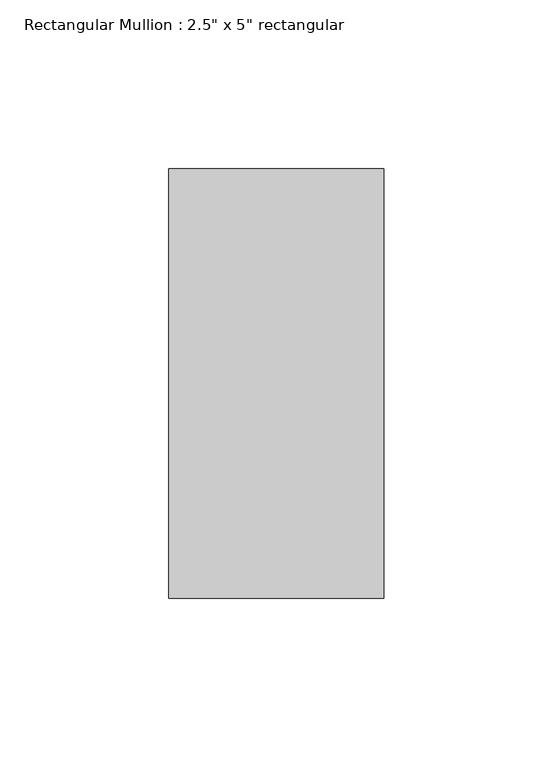
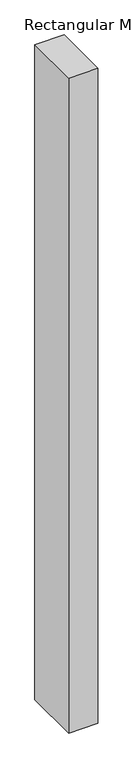
"""IFC4 building model written with IfcOpenShell, lengths in millimetres: member geometry."""

from ifc_helpers import new_model, si_unit, frame, origin, place, context, project, spatial, polyline, outline, extrude, source, transform, mapped, element, save


def member_9c2f0336(model_context):
    return source(origin(), model_context, "Body", "SweptSolid", [
        extrude(outline(polyline([(0.0, 63.5), (0.0, -63.5), (-63.5, -63.5), (-63.5, 63.5), (0.0, 63.5)])), frame((0.0, 0.0, -1506.17602), z_axis=(0.0, 0.0, 1.0), x_axis=(1.0, 0.0, 0.0)), (0.0, 0.0, 1.0), 1506.17602),
    ])


if __name__ == "__main__":
    model = new_model("IFC4")
    model_context = context("Model", 3, world=origin())
    ifc_project = project(units=[si_unit("LENGTHUNIT", "METRE", prefix="MILLI")], contexts=[model_context])
    site = spatial("IfcSite", under=ifc_project)
    building = spatial("IfcBuilding", under=site)
    placement = place(None, origin())
    member_shape = member_9c2f0336(model_context)
    element("IfcMember", 1, ObjectType="Rectangular Mullion : 2.5\" x 5\" rectangular", at=placement, inside=building, context=model_context, shape_type="MappedRepresentation", body=[
        mapped(member_shape, transform((0.0, 0.0, 0.0), x_axis=(1.0, 0.0, 0.0), y_axis=(0.0, 1.0, 0.0), z_axis=(0.0, 0.0, 1.0))),
    ])
    save(model, "model.ifc")

# Revit data of these elements
# Type "Rectangular Mullion : 2.5\" x 5\" rectangular"
#   built-in parameter 1007304 = 0.416667 (stored number, unit not read)
#   built-in parameter 1007301 = 0.104167 (stored number, unit not read)
#   built-in parameter 1007300 = 0.104167 (stored number, unit not read)
# Element 1 (IfcMember, "Rectangular Mullion : 2.5\" x 5\" rectangular")
#   Materials on its faces: "Aluminum"
# Materials
#   "Aluminum": class "Metal", colour RGB 247 247 247, transparency 0, Description = "Aluminum 6061", Cost = 0
